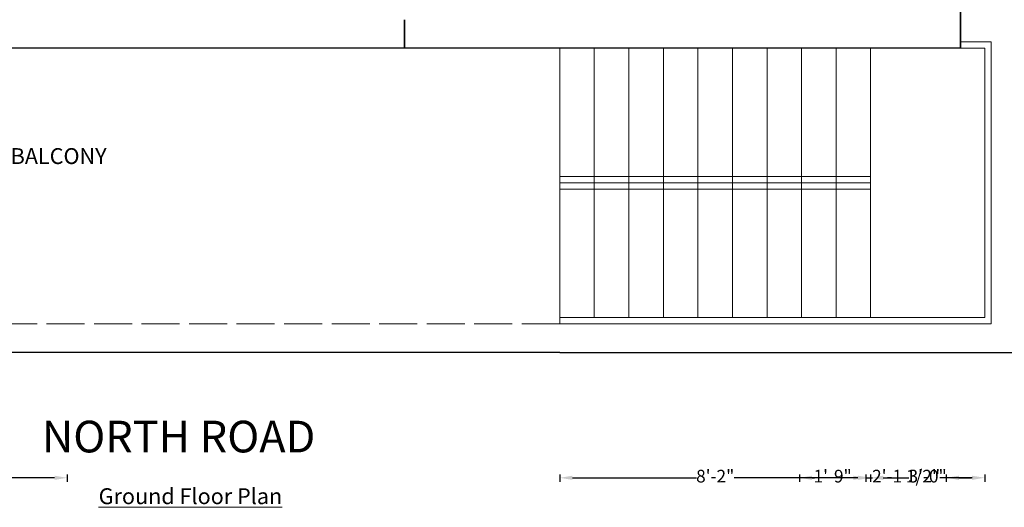
# Model space of a CAD drawing. Units: inches. Extents: x -638 to 186, y -762 to 59.
# Tile 2 of 31: x -287 to 24, y -762 to -608. Entities that reach past the tile are written whole.
import ezdxf

# ---------------------------------------------------------------- set-up
doc = ezdxf.new("R2010")
doc.units = ezdxf.units.IN
doc.linetypes.add('ACAD_ISO02W100', pattern=[15, 12, -3])
for name, color, linetype, lineweight in [('A-ANNO-DIMS', 2, 'Continuous', 18), ('A-AREA-IDEN', 1, 'Continuous', 18), ('A-FLOR-EDGE', 1, 'Continuous', 25), ('A-FLOR-OVHD', 1, 'ACAD_ISO02W100', 18), ('A-FLOR-STRS', 1, 'Continuous', 18), ('C-PROP', 7, 'Continuous', 25), ('txt', 7, 'Continuous', 18), ('wall', 7, 'Continuous', 35)]:
    doc.layers.add(name, color=color, linetype=linetype, lineweight=lineweight)
doc.styles.get("Standard").update_dxf_attribs({"font": 'arial.ttf'})
doc.dimstyles.new('ISO-25', dxfattribs={"dimtxt": 4, "dimasz": 4, "dimexe": 1.25, "dimexo": 0.625, "dimtad": 0, "dimlunit": 4, "dimtxsty": 'Standard', "dimcen": 2.5, "dimclrt": 256, "dimadec": 0, "dimazin": 0, "dimtfac": 1, "dimtmove": 0, "dimatfit": 3, "dimfxl": 1, "dimfxlon": 1, "dimarcsym": 0})

# ---------------------------------------------------------------- blocks, each defined once
blk = doc.blocks.new('*D12')
at = {"layer": 'A-ANNO-DIMS', "color": 0, "lineweight": -2, "transparency": 16777216}
for p, q in [((45.29, -615.03), (47.54, -615.03)), ((46.29, -625.03), (46.29, -645.66)), ((46.29, -694.03), (46.29, -673.41)), ((45.29, -704.03), (47.54, -704.03))]:
    blk.add_line(p, q, dxfattribs=at)
at = {"layer": 'A-ANNO-DIMS', "color": 0, "lineweight": 30, "transparency": 16777216}
for points in [[(44.62, -625.03), (47.95, -625.03), (46.29, -615.03)], [(44.62, -694.03), (47.95, -694.03), (46.29, -704.03)]]:
    blk.add_solid(points, dxfattribs=at)
at = {"layer": 'Defpoints', "color": 0, "lineweight": 30, "transparency": 16777216}
for p in [(20.08, -615.03), (20.08, -704.03), (46.29, -704.03)]:
    blk.add_point(p, dxfattribs=at)
at = {"layer": 'A-ANNO-DIMS', "color": 0, "transparency": 16777216, "insert": (46.29, -659.53), "char_height": 10, "attachment_point": 5, "rotation": 90}
blk.add_mtext('7\'-5"', dxfattribs=at)
blk = doc.blocks.new('*D14')
at = {"layer": 'A-ANNO-DIMS', "color": 0, "lineweight": -2, "transparency": 16777216}
for p, q in [((45.41, -42.03), (47.66, -42.03)), ((46.41, -52.03), (46.41, -307.65)), ((46.41, -607.03), (46.41, -351.42)), ((45.41, -617.03), (47.66, -617.03))]:
    blk.add_line(p, q, dxfattribs=at)
at = {"layer": 'A-ANNO-DIMS', "color": 0, "lineweight": 30, "transparency": 16777216}
for points in [[(44.74, -52.03), (48.08, -52.03), (46.41, -42.03)], [(44.74, -607.03), (48.08, -607.03), (46.41, -617.03)]]:
    blk.add_solid(points, dxfattribs=at)
at = {"layer": 'Defpoints', "color": 0, "lineweight": 30, "transparency": 16777216}
for p in [(10.47, -42.03), (10.47, -617.03), (46.41, -617.03)]:
    blk.add_point(p, dxfattribs=at)
at = {"layer": 'A-ANNO-DIMS', "color": 0, "transparency": 16777216, "insert": (46.41, -329.53), "char_height": 10, "attachment_point": 5, "rotation": 90}
blk.add_mtext('47\'-11"', dxfattribs=at)
blk = doc.blocks.new('*D15')
at = {"layer": 'A-ANNO-DIMS', "color": 0, "lineweight": -2, "transparency": 16777216}
for p, q in [((69.33, -24.03), (71.58, -24.03)), ((70.33, -34.03), (70.33, -350.73)), ((70.33, -703.03), (70.33, -386.33)), ((69.33, -713.03), (71.58, -713.03))]:
    blk.add_line(p, q, dxfattribs=at)
at = {"layer": 'A-ANNO-DIMS', "color": 0, "lineweight": 30, "transparency": 16777216}
for points in [[(68.66, -34.03), (72, -34.03), (70.33, -24.03)], [(68.66, -703.03), (72, -703.03), (70.33, -713.03)]]:
    blk.add_solid(points, dxfattribs=at)
at = {"layer": 'Defpoints', "color": 0, "lineweight": 30, "transparency": 16777216}
for p in [(-24.67, -24.03), (-10.56, -713.03), (70.33, -713.03)]:
    blk.add_point(p, dxfattribs=at)
at = {"layer": 'A-ANNO-DIMS', "color": 0, "transparency": 16777216, "insert": (70.33, -368.53), "char_height": 10, "attachment_point": 5, "rotation": 90}
blk.add_mtext('57\'-5"', dxfattribs=at)
blk = doc.blocks.new('*D35')
at = {"layer": 'A-ANNO-DIMS', "color": 0, "lineweight": -2, "transparency": 16777216}
for p, q in [((-116.04, -751.58), (-116.04, -753.83)), ((-17.92, -751.58), (-17.92, -753.83)), ((-112.04, -752.58), (-72.93, -752.58)), ((-21.92, -752.58), (-61.04, -752.58))]:
    blk.add_line(p, q, dxfattribs=at)
at = {"layer": 'A-ANNO-DIMS', "color": 0, "lineweight": 30, "transparency": 16777216}
for points in [[(-112.04, -751.92), (-112.04, -753.25), (-116.04, -752.58)], [(-21.92, -751.92), (-21.92, -753.25), (-17.92, -752.58)]]:
    blk.add_solid(points, dxfattribs=at)
at = {"layer": 'Defpoints', "color": 0, "lineweight": 30, "transparency": 16777216}
for p in [(-17.92, -702.03), (-116.04, -704.03), (-17.92, -752.58)]:
    blk.add_point(p, dxfattribs=at)
at = {"layer": 'A-ANNO-DIMS', "transparency": 16777216, "insert": (-66.98, -752.58), "char_height": 4, "attachment_point": 5}
blk.add_mtext('8\'-2"', dxfattribs=at)
blk = doc.blocks.new('*D36')
at = {"layer": 'A-ANNO-DIMS', "color": 0, "lineweight": -2, "transparency": 16777216}
for p, q in [((-17.92, -751.58), (-17.92, -753.83)), ((18.08, -751.58), (18.08, -753.83)), ((-13.92, -752.58), (-5.86, -752.58)), ((14.08, -752.58), (6.02, -752.58))]:
    blk.add_line(p, q, dxfattribs=at)
at = {"layer": 'A-ANNO-DIMS', "color": 0, "lineweight": 30, "transparency": 16777216}
for points in [[(-13.92, -751.92), (-13.92, -753.25), (-17.92, -752.58)], [(14.08, -751.92), (14.08, -753.25), (18.08, -752.58)]]:
    blk.add_solid(points, dxfattribs=at)
at = {"layer": 'Defpoints', "color": 0, "lineweight": 30, "transparency": 16777216}
for p in [(-17.92, -702.03), (18.08, -704.03), (18.08, -752.58)]:
    blk.add_point(p, dxfattribs=at)
at = {"layer": 'A-ANNO-DIMS', "transparency": 16777216, "insert": (0.08, -752.58), "char_height": 4, "attachment_point": 5}
blk.add_mtext('3\'-0"', dxfattribs=at)
blk = doc.blocks.new('*D39')
at = {"layer": 'A-ANNO-DIMS', "color": 0, "lineweight": -2, "transparency": 16777216}
for p, q in [((-344.53, -751.58), (-344.53, -753.83)), ((-271.53, -751.58), (-271.53, -753.83)), ((-340.53, -752.58), (-313.98, -752.58)), ((-275.53, -752.58), (-302.07, -752.58))]:
    blk.add_line(p, q, dxfattribs=at)
at = {"layer": 'A-ANNO-DIMS', "color": 0, "lineweight": 30, "transparency": 16777216}
for points in [[(-340.53, -751.92), (-340.53, -753.25), (-344.53, -752.58)], [(-275.53, -751.92), (-275.53, -753.25), (-271.53, -752.58)]]:
    blk.add_solid(points, dxfattribs=at)
at = {"layer": 'Defpoints', "color": 0, "lineweight": 30, "transparency": 16777216}
for p in [(-344.53, -214.53), (-271.53, -214.53), (-271.53, -752.58)]:
    blk.add_point(p, dxfattribs=at)
at = {"layer": 'A-ANNO-DIMS', "transparency": 16777216, "insert": (-308.03, -752.58), "char_height": 4, "attachment_point": 5}
blk.add_mtext('6\'-1"', dxfattribs=at)
blk = doc.blocks.new('*D51')
at = {"layer": 'A-ANNO-DIMS', "color": 0, "lineweight": -2, "transparency": 16777216}
for p, q in [((-40.41, -751.58), (-40.41, -753.83)), ((-19.41, -751.58), (-19.41, -753.83)), ((-36.41, -752.58), (-35.66, -752.58)), ((-23.41, -752.58), (-24.15, -752.58))]:
    blk.add_line(p, q, dxfattribs=at)
at = {"layer": 'A-ANNO-DIMS', "color": 0, "lineweight": 30, "transparency": 16777216}
for points in [[(-36.41, -751.92), (-36.41, -753.25), (-40.41, -752.58)], [(-23.41, -751.92), (-23.41, -753.25), (-19.41, -752.58)]]:
    blk.add_solid(points, dxfattribs=at)
at = {"layer": 'Defpoints', "color": 0, "lineweight": 30, "transparency": 16777216}
for p in [(-40.41, -608.03), (-19.41, -608.03), (-19.41, -752.58)]:
    blk.add_point(p, dxfattribs=at)
at = {"layer": 'A-ANNO-DIMS', "transparency": 16777216, "insert": (-29.91, -752.58), "char_height": 4, "attachment_point": 5}
blk.add_mtext('1\'-9"', dxfattribs=at)
blk = doc.blocks.new('*D52')
at = {"layer": 'A-ANNO-DIMS', "color": 0, "lineweight": -2, "transparency": 16777216}
for p, q in [((-630.93, -580.03), (-633.18, -580.03)), ((-631.93, -584.03), (-631.93, -588.06)), ((-631.93, -604.03), (-631.93, -600.01)), ((-630.93, -608.03), (-633.18, -608.03))]:
    blk.add_line(p, q, dxfattribs=at)
at = {"layer": 'A-ANNO-DIMS', "color": 0, "lineweight": 30, "transparency": 16777216}
for points in [[(-632.59, -584.03), (-631.26, -584.03), (-631.93, -580.03)], [(-632.59, -604.03), (-631.26, -604.03), (-631.93, -608.03)]]:
    blk.add_solid(points, dxfattribs=at)
at = {"layer": 'Defpoints', "color": 0, "lineweight": 30, "transparency": 16777216}
for p in [(-29.91, -580.03), (-631.93, -608.03), (-40.41, -608.03)]:
    blk.add_point(p, dxfattribs=at)
at = {"layer": 'A-ANNO-DIMS', "transparency": 16777216, "insert": (-631.93, -594.03), "char_height": 4, "attachment_point": 5, "rotation": 90}
blk.add_mtext('2\'-4"', dxfattribs=at)
blk = doc.blocks.new('*D53')
at = {"layer": 'A-ANNO-DIMS', "color": 0, "lineweight": -2, "transparency": 16777216}
for p, q in [((-19.41, -751.58), (-19.41, -753.83)), ((5.97, -751.58), (5.97, -753.83)), ((-23.41, -752.58), (-27.41, -752.58)), ((-19.41, -752.58), (-17.35, -752.58)), ((5.97, -752.58), (3.92, -752.58)), ((9.97, -752.58), (13.97, -752.58))]:
    blk.add_line(p, q, dxfattribs=at)
at = {"layer": 'A-ANNO-DIMS', "color": 0, "lineweight": 30, "transparency": 16777216}
for points in [[(-23.41, -751.92), (-23.41, -753.25), (-19.41, -752.58)], [(9.97, -751.92), (9.97, -753.25), (5.97, -752.58)]]:
    blk.add_solid(points, dxfattribs=at)
at = {"layer": 'Defpoints', "color": 0, "lineweight": 30, "transparency": 16777216}
for p in [(-19.41, -608.03), (5.97, -608.03), (5.97, -752.58)]:
    blk.add_point(p, dxfattribs=at)
at = {"layer": 'A-ANNO-DIMS', "transparency": 16777216, "insert": (-6.72, -752.58), "char_height": 4, "attachment_point": 5}
blk.add_mtext('2\'-1 1/2"', dxfattribs=at)

msp = doc.modelspace()

# ---------------------------------------------------------------- linework, layer by layer
at = {"layer": 'A-FLOR-EDGE'}
for p, q in [((-165.026, -617.033), (-413.526, -617.033)), ((10.474, -617.033), (-165.026, -617.033))]:
    msp.add_line(p, q, dxfattribs=at)
at = {"layer": 'A-FLOR-OVHD'}
msp.add_line((-116.044, -704.033), (-455.526, -704.033), dxfattribs=at)
at = {"layer": 'A-FLOR-STRS'}
for p, q in [((10.474, -615.033), (18.081, -615.033)), ((18.081, -615.033), (20.081, -615.033)), ((20.081, -615.033), (20.081, -704.033)), ((-116.044, -702.033), (-116.044, -617.033)), ((-116.044, -617.033), (-116.044, -702.033)), ((-105.142, -617.033), (-105.142, -702.033)), ((-94.239, -617.033), (-94.239, -702.033)), ((-83.336, -617.033), (-83.336, -702.033)), ((-72.433, -617.033), (-72.433, -702.033)), ((-61.53, -617.033), (-61.53, -702.033)), ((-50.627, -617.033), (-50.627, -702.033)), ((-39.724, -617.033), (-39.724, -702.033)), ((-28.821, -617.033), (-28.821, -702.033)), ((-17.919, -617.033), (-17.919, -702.033)), ((10.474, -617.033), (18.081, -617.033)), ((18.081, -617.033), (18.081, -702.033)), ((-17.919, -657.533), (-116.044, -657.533)), ((-17.919, -659.533), (-116.044, -659.533)), ((-17.919, -661.533), (-116.044, -661.533)), ((18.081, -702.033), (-116.044, -702.033)), ((-116.044, -704.033), (-116.044, -702.033)), ((18.081, -704.033), (-116.044, -704.033)), ((18.081, -704.033), (20.081, -704.033))]:
    msp.add_line(p, q, dxfattribs=at)
at = {"layer": 'C-PROP'}
for q in [(-455.526, -713.033), (28.474, -713.033)]:
    msp.add_line((-116.044, -713.033), q, dxfattribs=at)
at = {"layer": 'wall'}
for p, q in [((10.474, -42.033), (10.474, -617.033)), ((-165.026, -608.033), (-165.026, -617.033))]:
    msp.add_line(p, q, dxfattribs=at)

# ---------------------------------------------------------------- texts
at = {"layer": 'A-AREA-IDEN', "insert": (-305.974, -648.566), "char_height": 5, "attachment_point": 1}
msp.add_mtext_dynamic_manual_height_columns('6\'-6" BALCONY', width=109.8979, gutter_width=12.5, heights=[0], dxfattribs=at)
at = {"layer": 'txt', "attachment_point": 1}
for s, width, insert, char_height in [('NORTH ROAD', 268.39333, (-279.48, -734.574), 10), ('{\\LGround Floor Plan}', 192.28251, (-261.594, -755.891), 5)]:
    msp.add_mtext_dynamic_manual_height_columns(s, width=width, gutter_width=12.5, heights=[0], dxfattribs=dict(at, insert=insert, char_height=char_height))

# ---------------------------------------------------------------- dimensions: what is measured, and where the dimension line sits
at = {"layer": 'A-ANNO-DIMS'}
for base, p1, p2, override, picture, middle in [((70.331, -713.033), (-24.669, -24.033), (-10.563, -713.033), {"dimtxt": 10, "dimasz": 10, "dimclrd": 0, "dimclre": 0, "dimclrt": 0}, '*D15', (70.331, -368.533)), ((46.411, -617.033), (10.474, -42.033), (10.474, -617.033), {"dimtxt": 10, "dimasz": 10, "dimclrd": 0, "dimclre": 0, "dimclrt": 0}, '*D14', (46.411, -329.533)), ((-631.926, -608.033), (-29.908, -580.033), (-40.408, -608.033), {"dimdec": 1, "dimlfac": 1, "dimrnd": 0, "dimzin": 1, "dimdsep": 46, "dimlunit": 4, "dimfrac": 2}, '*D52', (-631.926, -594.033)), ((46.286, -704.033), (20.081, -615.033), (20.081, -704.033), {"dimtxt": 10, "dimasz": 10, "dimclrd": 0, "dimclre": 0, "dimclrt": 0}, '*D12', (46.286, -659.533))]:
    dim = msp.add_linear_dim(base=base, p1=p1, p2=p2, angle=90, dimstyle='ISO-25', override=override, dxfattribs=at)
    dim.commit()
    dim.dimension.update_dxf_attribs({"geometry": picture, "text_midpoint": middle})
for base, p1, p2, picture, middle in [((-271.526, -752.583), (-344.526, -214.533), (-271.526, -214.533), '*D39', (-308.026, -752.583)), ((-19.408, -752.583), (-40.408, -608.033), (-19.408, -608.033), '*D51', (-29.908, -752.583)), ((5.974, -752.583), (-19.408, -608.033), (5.974, -608.033), '*D53', (-6.717, -752.583)), ((-17.919, -752.583), (-116.044, -704.033), (-17.919, -702.033), '*D35', (-66.982, -752.583)), ((18.081, -752.583), (-17.919, -702.033), (18.081, -704.033), '*D36', (0.081, -752.583))]:
    dim = msp.add_linear_dim(base=base, p1=p1, p2=p2, dimstyle='ISO-25', override={"dimdec": 1, "dimlfac": 1, "dimrnd": 0, "dimzin": 1, "dimdsep": 46, "dimlunit": 4, "dimfrac": 2}, dxfattribs=at)
    dim.commit()
    dim.dimension.update_dxf_attribs({"geometry": picture, "text_midpoint": middle})

doc.saveas('drawing.dxf')
